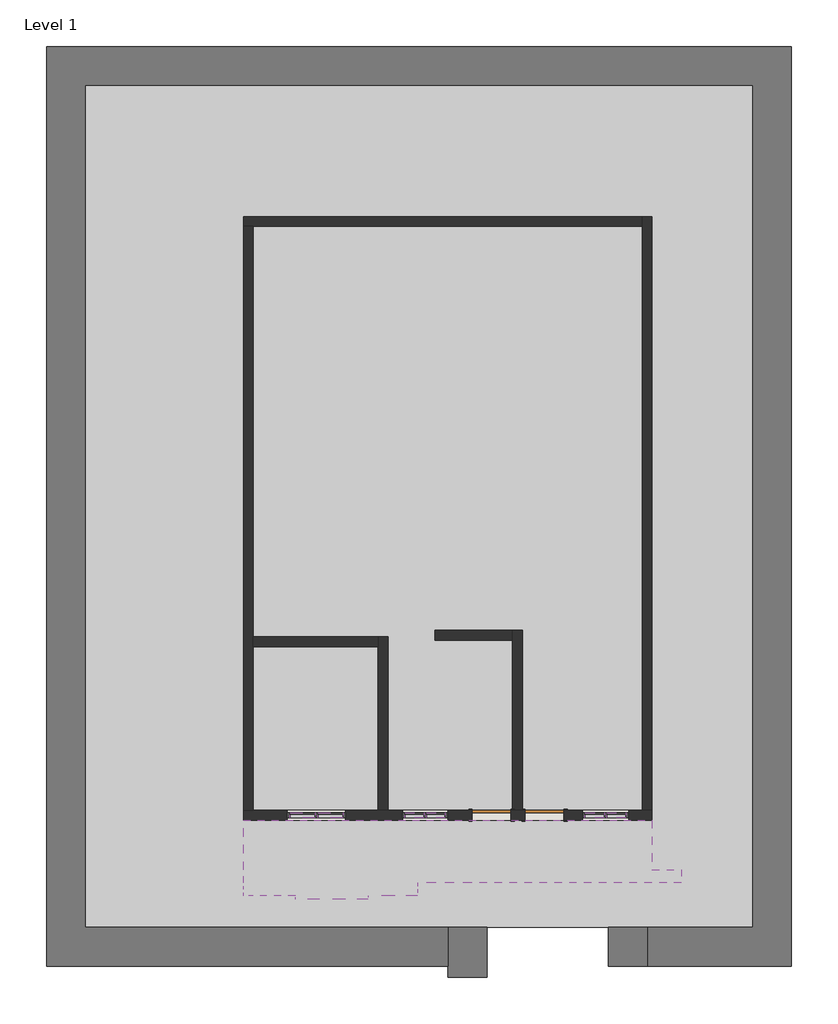
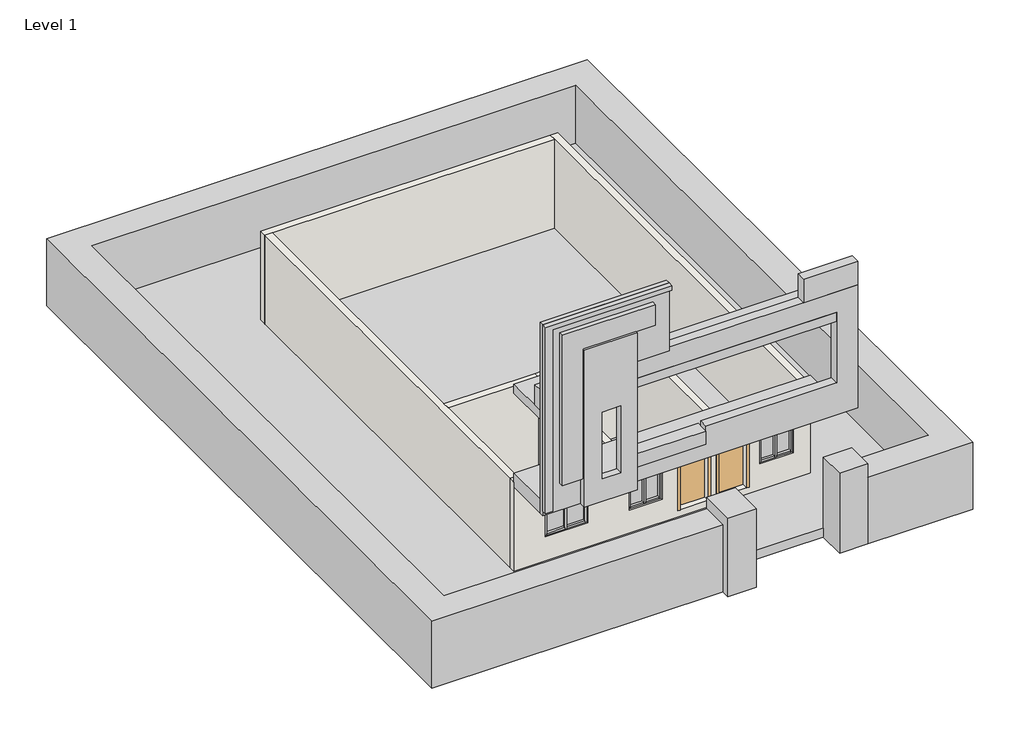
# One storey: 21 members, 8 walls, 6 plates, 3 proxies, 2 doors.
"""IFC4 building model written with IfcOpenShell, lengths in millimetres."""

from ifc_helpers import new_model, si_unit, origin, origin_with_axes, place, context, project, spatial, polyline, outline, extrude, faceted_brep, transform, mapped, element, save
from components import generic_models_1_generic_models_1_a3900748, generic_models_2_generic_models_2_88d393e9, generic_models_3_generic_models_3_c69b0eb2, door_a90ba1ad, door_0ca8825f, member_e5d39754, member_25a9efec, member_dca25542, member_6fb4a552, member_194281bb, member_24084ae4, member_969ca954, member_fe23b6ba, member_92f7bfeb, system_panel_glazed_4c12f6d8, system_panel_glazed_673a7a74, system_panel_glazed_2348052a

model = new_model("IFC4")

# Units and contexts
model_context = context("Model", 3, world=origin())
ifc_project = project(units=[si_unit("LENGTHUNIT", "METRE", prefix="MILLI")], contexts=[model_context])

# Site, building, storey
site = spatial("IfcSite", under=ifc_project)
building = spatial("IfcBuilding", under=site)
storey = spatial("IfcBuildingStorey", under=building, Name="Level 1", Elevation=0.0)

# Proxies
placement = place(None, origin())
generic_models_1_generic_models_1_shape = generic_models_1_generic_models_1_a3900748(model_context)
element("IfcBuildingElementProxy", 1, Name="Generic Models 1 : Generic Models 1", ObjectType="Generic Models 1 : Generic Models 1", at=placement, inside=storey, context=model_context, shape_type="MappedRepresentation", body=[
    mapped(generic_models_1_generic_models_1_shape, transform((0.0, 0.0, 0.0), x_axis=(1.0, 0.0, 0.0), y_axis=(0.0, 1.0, 0.0), z_axis=(0.0, 0.0, 1.0))),
])
generic_models_2_generic_models_2_shape = generic_models_2_generic_models_2_88d393e9(model_context)
element("IfcBuildingElementProxy", 2, Name="Generic Models 2 : Generic Models 2", ObjectType="Generic Models 2 : Generic Models 2", at=placement, inside=storey, context=model_context, shape_type="MappedRepresentation", body=[
    mapped(generic_models_2_generic_models_2_shape, transform((0.0, 0.0, 0.0), x_axis=(1.0, 0.0, 0.0), y_axis=(0.0, 1.0, 0.0), z_axis=(0.0, 0.0, 1.0))),
])
generic_models_3_generic_models_3_shape = generic_models_3_generic_models_3_c69b0eb2(model_context)
element("IfcBuildingElementProxy", 3, Name="Generic Models 3 : Generic Models 3", ObjectType="Generic Models 3 : Generic Models 3", at=placement, inside=storey, context=model_context, shape_type="MappedRepresentation", body=[
    mapped(generic_models_3_generic_models_3_shape, transform((0.0, 0.0, 0.0), x_axis=(1.0, 0.0, 0.0), y_axis=(0.0, 1.0, 0.0), z_axis=(0.0, 0.0, 1.0))),
])

# Doors
door_shape = door_a90ba1ad(model_context)
element("IfcDoor", 4, ObjectType="Single-Flush : 36\" x 84\"", at=placement, inside=storey, context=model_context, shape_type="MappedRepresentation", body=[
    mapped(door_shape, transform((-11559.1094994, -14629.3805842, 228.6), x_axis=(-1.0, 0.0, 0.0), y_axis=(0.0, -1.0, 0.0), z_axis=(0.0, 0.0, 1.0))),
])
door_2_shape = door_0ca8825f(model_context)
element("IfcDoor", 5, ObjectType="Single-Flush : 36\" x 84\"", at=placement, inside=storey, context=model_context, shape_type="MappedRepresentation", body=[
    mapped(door_2_shape, transform((-12803.7094994, -14629.3805842, 228.6), x_axis=(1.0, 0.0, 0.0), y_axis=(0.0, 1.0, 0.0), z_axis=(0.0, 0.0, 1.0))),
])

# Members
member_shape = member_e5d39754(model_context)
element("IfcMember", 6, ObjectType="Rectangular Mullion : 2.5\" x 5\" rectangular", at=placement, inside=storey, context=model_context, shape_type="MappedRepresentation", body=[
    mapped(member_shape, transform((-16950.2594994, -14629.3805842, 2460.3329458), x_axis=(0.0, 0.0, 1.0), y_axis=(0.0, -1.0, 0.0), z_axis=(1.0, 0.0, 0.0))),
])
element("IfcMember", 7, ObjectType="Rectangular Mullion : 2.5\" x 5\" rectangular", at=placement, inside=storey, context=model_context, shape_type="MappedRepresentation", body=[
    mapped(member_shape, transform((-16296.2094994, -14629.3805842, 2460.3329458), x_axis=(0.0, 0.0, 1.0), y_axis=(0.0, -1.0, 0.0), z_axis=(1.0, 0.0, 0.0))),
])
member_2_shape = member_25a9efec(model_context)
element("IfcMember", 8, ObjectType="Rectangular Mullion : 2.5\" x 5\" rectangular", at=placement, inside=storey, context=model_context, shape_type="MappedRepresentation", body=[
    mapped(member_2_shape, transform((-16918.5094994, -14629.3805842, 816.0272948), x_axis=(1.0, 0.0, 0.0), y_axis=(0.0, -1.0, 0.0), z_axis=(0.0, 0.0, -1.0))),
])
element("IfcMember", 9, ObjectType="Rectangular Mullion : 2.5\" x 5\" rectangular", at=placement, inside=storey, context=model_context, shape_type="MappedRepresentation", body=[
    mapped(member_shape, transform((-16886.7594994, -14629.3805842, 816.0272948), x_axis=(0.0, 0.0, -1.0), y_axis=(0.0, -1.0, 0.0), z_axis=(-1.0, 0.0, 0.0))),
])
element("IfcMember", 10, ObjectType="Rectangular Mullion : 2.5\" x 5\" rectangular", at=placement, inside=storey, context=model_context, shape_type="MappedRepresentation", body=[
    mapped(member_shape, transform((-17540.8094994, -14629.3805842, 816.0272948), x_axis=(0.0, 0.0, -1.0), y_axis=(0.0, -1.0, 0.0), z_axis=(-1.0, 0.0, 0.0))),
])
member_3_shape = member_dca25542(model_context)
element("IfcMember", 11, ObjectType="Rectangular Mullion : 2.5\" x 5\" rectangular", at=placement, inside=storey, context=model_context, shape_type="MappedRepresentation", body=[
    mapped(member_3_shape, transform((-17604.3094994, -14629.3805842, 2460.3329458), x_axis=(-1.0, 0.0, 0.0), y_axis=(0.0, -1.0, 0.0), z_axis=(0.0, 0.0, 1.0))),
])
element("IfcMember", 12, ObjectType="Rectangular Mullion : 2.5\" x 5\" rectangular", at=placement, inside=storey, context=model_context, shape_type="MappedRepresentation", body=[
    mapped(member_3_shape, transform((-16232.7094994, -14629.3805842, 816.0272948), x_axis=(1.0, 0.0, 0.0), y_axis=(0.0, -1.0, 0.0), z_axis=(0.0, 0.0, -1.0))),
])
member_4_shape = member_6fb4a552(model_context)
element("IfcMember", 13, ObjectType="Rectangular Mullion : 2.5\" x 5\" rectangular", at=placement, inside=storey, context=model_context, shape_type="MappedRepresentation", body=[
    mapped(member_4_shape, transform((-14397.5594994, -14629.3805842, 2430.1873422), x_axis=(0.0, 0.0, 1.0), y_axis=(0.0, -1.0, 0.0), z_axis=(1.0, 0.0, 0.0))),
])
element("IfcMember", 14, ObjectType="Rectangular Mullion : 2.5\" x 5\" rectangular", at=placement, inside=storey, context=model_context, shape_type="MappedRepresentation", body=[
    mapped(member_4_shape, transform((-13895.9094994, -14629.3805842, 2430.1873422), x_axis=(0.0, 0.0, 1.0), y_axis=(0.0, -1.0, 0.0), z_axis=(1.0, 0.0, 0.0))),
])
member_5_shape = member_194281bb(model_context)
element("IfcMember", 15, ObjectType="Rectangular Mullion : 2.5\" x 5\" rectangular", at=placement, inside=storey, context=model_context, shape_type="MappedRepresentation", body=[
    mapped(member_5_shape, transform((-14365.8094994, -14629.3805842, 785.4534866), x_axis=(1.0, 0.0, 0.0), y_axis=(0.0, -1.0, 0.0), z_axis=(0.0, 0.0, -1.0))),
])
element("IfcMember", 16, ObjectType="Rectangular Mullion : 2.5\" x 5\" rectangular", at=placement, inside=storey, context=model_context, shape_type="MappedRepresentation", body=[
    mapped(member_4_shape, transform((-14334.0594994, -14629.3805842, 785.4534866), x_axis=(0.0, 0.0, -1.0), y_axis=(0.0, -1.0, 0.0), z_axis=(-1.0, 0.0, 0.0))),
])
element("IfcMember", 17, ObjectType="Rectangular Mullion : 2.5\" x 5\" rectangular", at=placement, inside=storey, context=model_context, shape_type="MappedRepresentation", body=[
    mapped(member_4_shape, transform((-14835.7094994, -14629.3805842, 785.4534866), x_axis=(0.0, 0.0, -1.0), y_axis=(0.0, -1.0, 0.0), z_axis=(-1.0, 0.0, 0.0))),
])
member_6_shape = member_24084ae4(model_context)
element("IfcMember", 18, ObjectType="Rectangular Mullion : 2.5\" x 5\" rectangular", at=placement, inside=storey, context=model_context, shape_type="MappedRepresentation", body=[
    mapped(member_6_shape, transform((-14899.2094994, -14629.3805842, 2430.1873422), x_axis=(-1.0, 0.0, 0.0), y_axis=(0.0, -1.0, 0.0), z_axis=(0.0, 0.0, 1.0))),
])
element("IfcMember", 19, ObjectType="Rectangular Mullion : 2.5\" x 5\" rectangular", at=placement, inside=storey, context=model_context, shape_type="MappedRepresentation", body=[
    mapped(member_6_shape, transform((-13832.4094994, -14629.3805842, 785.4534866), x_axis=(1.0, 0.0, 0.0), y_axis=(0.0, -1.0, 0.0), z_axis=(0.0, 0.0, -1.0))),
])
member_7_shape = member_969ca954(model_context)
element("IfcMember", 20, ObjectType="Rectangular Mullion : 2.5\" x 5\" rectangular", at=placement, inside=storey, context=model_context, shape_type="MappedRepresentation", body=[
    mapped(member_7_shape, transform((-10155.7594994, -14629.3805842, 2382.0013914), x_axis=(0.0, 0.0, 1.0), y_axis=(0.0, -1.0, 0.0), z_axis=(1.0, 0.0, 0.0))),
])
element("IfcMember", 21, ObjectType="Rectangular Mullion : 2.5\" x 5\" rectangular", at=placement, inside=storey, context=model_context, shape_type="MappedRepresentation", body=[
    mapped(member_7_shape, transform((-9641.4094994, -14629.3805842, 2382.0013914), x_axis=(0.0, 0.0, 1.0), y_axis=(0.0, -1.0, 0.0), z_axis=(1.0, 0.0, 0.0))),
])
member_8_shape = member_fe23b6ba(model_context)
element("IfcMember", 22, ObjectType="Rectangular Mullion : 2.5\" x 5\" rectangular", at=placement, inside=storey, context=model_context, shape_type="MappedRepresentation", body=[
    mapped(member_8_shape, transform((-10124.0094994, -14629.3805842, 889.778584), x_axis=(1.0, 0.0, 0.0), y_axis=(0.0, -1.0, 0.0), z_axis=(0.0, 0.0, -1.0))),
])
element("IfcMember", 23, ObjectType="Rectangular Mullion : 2.5\" x 5\" rectangular", at=placement, inside=storey, context=model_context, shape_type="MappedRepresentation", body=[
    mapped(member_7_shape, transform((-10092.2594994, -14629.3805842, 889.778584), x_axis=(0.0, 0.0, -1.0), y_axis=(0.0, -1.0, 0.0), z_axis=(-1.0, 0.0, 0.0))),
])
element("IfcMember", 24, ObjectType="Rectangular Mullion : 2.5\" x 5\" rectangular", at=placement, inside=storey, context=model_context, shape_type="MappedRepresentation", body=[
    mapped(member_7_shape, transform((-10606.6094994, -14629.3805842, 889.778584), x_axis=(0.0, 0.0, -1.0), y_axis=(0.0, -1.0, 0.0), z_axis=(-1.0, 0.0, 0.0))),
])
member_9_shape = member_92f7bfeb(model_context)
element("IfcMember", 25, ObjectType="Rectangular Mullion : 2.5\" x 5\" rectangular", at=placement, inside=storey, context=model_context, shape_type="MappedRepresentation", body=[
    mapped(member_9_shape, transform((-10670.1094994, -14629.3805842, 2382.0013914), x_axis=(-1.0, 0.0, 0.0), y_axis=(0.0, -1.0, 0.0), z_axis=(0.0, 0.0, 1.0))),
])
element("IfcMember", 26, ObjectType="Rectangular Mullion : 2.5\" x 5\" rectangular", at=placement, inside=storey, context=model_context, shape_type="MappedRepresentation", body=[
    mapped(member_9_shape, transform((-9577.9094994, -14629.3805842, 889.778584), x_axis=(1.0, 0.0, 0.0), y_axis=(0.0, -1.0, 0.0), z_axis=(0.0, 0.0, -1.0))),
])

# Plates
system_panel_glazed_shape = system_panel_glazed_4c12f6d8(model_context)
element("IfcPlate", 27, ObjectType="System Panel : Glazed", at=placement, inside=storey, context=model_context, shape_type="MappedRepresentation", body=[
    mapped(system_panel_glazed_shape, transform((-17245.5344994, -14629.3805842, 879.5272948), x_axis=(1.0, 0.0, 0.0), y_axis=(0.0, 1.0, 0.0), z_axis=(0.0, 0.0, 1.0))),
])
element("IfcPlate", 28, ObjectType="System Panel : Glazed", at=placement, inside=storey, context=model_context, shape_type="MappedRepresentation", body=[
    mapped(system_panel_glazed_shape, transform((-16591.4844994, -14629.3805842, 879.5272948), x_axis=(1.0, 0.0, 0.0), y_axis=(0.0, 1.0, 0.0), z_axis=(0.0, 0.0, 1.0))),
])
system_panel_glazed_2_shape = system_panel_glazed_673a7a74(model_context)
element("IfcPlate", 29, ObjectType="System Panel : Glazed", at=placement, inside=storey, context=model_context, shape_type="MappedRepresentation", body=[
    mapped(system_panel_glazed_2_shape, transform((-14616.6344994, -14629.3805842, 848.9534866), x_axis=(1.0, 0.0, 0.0), y_axis=(0.0, 1.0, 0.0), z_axis=(0.0, 0.0, 1.0))),
])
element("IfcPlate", 30, ObjectType="System Panel : Glazed", at=placement, inside=storey, context=model_context, shape_type="MappedRepresentation", body=[
    mapped(system_panel_glazed_2_shape, transform((-14114.9844994, -14629.3805842, 848.9534866), x_axis=(1.0, 0.0, 0.0), y_axis=(0.0, 1.0, 0.0), z_axis=(0.0, 0.0, 1.0))),
])
system_panel_glazed_3_shape = system_panel_glazed_2348052a(model_context)
element("IfcPlate", 31, ObjectType="System Panel : Glazed", at=placement, inside=storey, context=model_context, shape_type="MappedRepresentation", body=[
    mapped(system_panel_glazed_3_shape, transform((-10381.1844994, -14629.3805842, 953.278584), x_axis=(1.0, 0.0, 0.0), y_axis=(0.0, 1.0, 0.0), z_axis=(0.0, 0.0, 1.0))),
])
element("IfcPlate", 32, ObjectType="System Panel : Glazed", at=placement, inside=storey, context=model_context, shape_type="MappedRepresentation", body=[
    mapped(system_panel_glazed_3_shape, transform((-9866.8344994, -14629.3805842, 953.278584), x_axis=(1.0, 0.0, 0.0), y_axis=(0.0, 1.0, 0.0), z_axis=(0.0, 0.0, 1.0))),
])

# Walls
element("IfcWall", 33, ObjectType="9\"", at=placement, inside=storey, context=model_context, shape_type="Brep", body=[
    faceted_brep([(-18633.0094994, -14743.6805842, 0.0), (-9031.8094994, -14743.6805842, 0.0), (-9031.8094994, -14743.6805842, 3048.0), (-18633.0094994, -14743.6805842, 3048.0), (-11101.9094994, -14743.6805842, 228.6), (-12016.3094994, -14743.6805842, 228.6), (-12016.3094994, -14743.6805842, 2362.2), (-11101.9094994, -14743.6805842, 2362.2), (-13260.9094994, -14743.6805842, 228.6), (-13260.9094994, -14743.6805842, 2362.2), (-12346.5094994, -14743.6805842, 2362.2), (-12346.5094994, -14743.6805842, 228.6), (-10670.1094994, -14743.6805842, 889.778584), (-10670.1094994, -14743.6805842, 2382.0013914), (-9577.9094994, -14743.6805842, 2382.0013914), (-9577.9094994, -14743.6805842, 889.778584), (-14899.2094994, -14743.6805842, 785.4534866), (-14899.2094994, -14743.6805842, 2430.1873422), (-13832.4094994, -14743.6805842, 2430.1873422), (-13832.4094994, -14743.6805842, 785.4534866), (-17604.3094994, -14743.6805842, 816.0272948), (-17604.3094994, -14743.6805842, 2460.3329458), (-16232.7094994, -14743.6805842, 2460.3329458), (-16232.7094994, -14743.6805842, 816.0272948), (-9031.8094994, -14515.0805842, 0.0), (-9260.4094994, -14515.0805842, 0.0), (-12079.8094994, -14515.0805842, 0.0), (-12308.4094994, -14515.0805842, 0.0), (-15242.1094994, -14515.0805842, 0.0), (-15470.7094994, -14515.0805842, 0.0), (-18404.4094994, -14515.0805842, 0.0), (-18633.0094994, -14515.0805842, 0.0), (-18633.0094994, -14515.0805842, 3048.0), (-18404.4094994, -14515.0805842, 3048.0), (-15470.7094994, -14515.0805842, 3048.0), (-15242.1094994, -14515.0805842, 3048.0), (-12308.4094994, -14515.0805842, 3048.0), (-12079.8094994, -14515.0805842, 3048.0), (-9260.4094994, -14515.0805842, 3048.0), (-9031.8094994, -14515.0805842, 3048.0), (-11101.9094994, -14515.0805842, 228.6), (-11101.9094994, -14515.0805842, 2362.2), (-12016.3094994, -14515.0805842, 2362.2), (-12016.3094994, -14515.0805842, 228.6), (-13260.9094994, -14515.0805842, 228.6), (-12346.5094994, -14515.0805842, 228.6), (-12346.5094994, -14515.0805842, 2362.2), (-13260.9094994, -14515.0805842, 2362.2), (-10670.1094994, -14515.0805842, 2382.0013914), (-10670.1094994, -14515.0805842, 889.778584), (-9577.9094994, -14515.0805842, 889.778584), (-9577.9094994, -14515.0805842, 2382.0013914), (-14899.2094994, -14515.0805842, 2430.1873422), (-14899.2094994, -14515.0805842, 785.4534866), (-13832.4094994, -14515.0805842, 785.4534866), (-13832.4094994, -14515.0805842, 2430.1873422), (-17604.3094994, -14515.0805842, 2460.3329458), (-17604.3094994, -14515.0805842, 816.0272948), (-16232.7094994, -14515.0805842, 816.0272948), (-16232.7094994, -14515.0805842, 2460.3329458)], [[[0, 1, 2, 3], [4, 5, 6, 7], [8, 9, 10, 11], [12, 13, 14, 15], [16, 17, 18, 19], [20, 21, 22, 23]], [[24, 25, 26, 27, 28, 29, 30, 31, 32, 33, 34, 35, 36, 37, 38, 39], [40, 41, 42, 43], [44, 45, 46, 47], [48, 49, 50, 51], [52, 53, 54, 55], [56, 57, 58, 59]], [[1, 0, 31, 30, 29, 28, 27, 26, 25, 24]], [[3, 2, 39, 38, 37, 36, 35, 34, 33, 32]], [[2, 1, 24, 39]], [[0, 3, 32, 31]], [[5, 4, 40, 43]], [[6, 5, 43, 42]], [[7, 6, 42, 41]], [[4, 7, 41, 40]], [[45, 44, 8, 11]], [[46, 45, 11, 10]], [[47, 46, 10, 9]], [[44, 47, 9, 8]], [[12, 49, 48, 13]], [[13, 48, 51, 14]], [[14, 51, 50, 15]], [[49, 12, 15, 50]], [[52, 17, 16, 53]], [[17, 52, 55, 18]], [[18, 55, 54, 19]], [[53, 16, 19, 54]], [[56, 21, 20, 57]], [[21, 56, 59, 22]], [[22, 59, 58, 23]], [[57, 20, 23, 58]]]),
])
element("IfcWall", 34, ObjectType="9\"", at=placement, inside=storey, context=model_context, shape_type="Brep", body=[
    faceted_brep([(-9031.8094994, -14515.0805842, 0.0), (-9031.8094994, -570.4805842, 0.0), (-9031.8094994, -570.4805842, 3048.0), (-9031.8094994, -14515.0805842, 3048.0), (-9260.4094994, -14515.0805842, 0.0), (-9260.4094994, -14515.0805842, 3048.0), (-9260.4094994, -799.0805842, 3048.0), (-9260.4094994, -570.4805842, 3048.0), (-9260.4094994, -570.4805842, 0.0), (-9260.4094994, -799.0805842, 0.0)], [[[0, 1, 2, 3]], [[4, 5, 6, 7, 8, 9]], [[1, 0, 4, 9, 8]], [[3, 2, 7, 6, 5]], [[0, 3, 5, 4]], [[2, 1, 8, 7]]]),
])
element("IfcWall", 35, ObjectType="9\"", at=placement, inside=storey, context=model_context, shape_type="Brep", body=[
    faceted_brep([(-9260.4094994, -570.4805842, 0.0), (-18633.0094994, -570.4805842, 0.0), (-18633.0094994, -570.4805842, 3048.0), (-9260.4094994, -570.4805842, 3048.0), (-9260.4094994, -799.0805842, 0.0), (-9260.4094994, -799.0805842, 3048.0), (-18404.4094994, -799.0805842, 3048.0), (-18633.0094994, -799.0805842, 3048.0), (-18633.0094994, -799.0805842, 0.0), (-18404.4094994, -799.0805842, 0.0)], [[[0, 1, 2, 3]], [[4, 5, 6, 7, 8, 9]], [[1, 0, 4, 9, 8]], [[3, 2, 7, 6, 5]], [[0, 3, 5, 4]], [[2, 1, 8, 7]]]),
])
element("IfcWall", 36, ObjectType="9\"", at=placement, inside=storey, context=model_context, shape_type="Brep", body=[
    faceted_brep([(-18633.0094994, -799.0805842, 0.0), (-18633.0094994, -14515.0805842, 0.0), (-18633.0094994, -14515.0805842, 3048.0), (-18633.0094994, -799.0805842, 3048.0), (-18404.4094994, -799.0805842, 0.0), (-18404.4094994, -799.0805842, 3048.0), (-18404.4094994, -10438.3805842, 3048.0), (-18404.4094994, -10666.9805842, 3048.0), (-18404.4094994, -14515.0805842, 3048.0), (-18404.4094994, -14515.0805842, 0.0), (-18404.4094994, -10666.9805842, 0.0), (-18404.4094994, -10438.3805842, 0.0)], [[[0, 1, 2, 3]], [[4, 5, 6, 7, 8, 9, 10, 11]], [[1, 0, 4, 11, 10, 9]], [[3, 2, 8, 7, 6, 5]], [[0, 3, 5, 4]], [[2, 1, 9, 8]]]),
])
element("IfcWall", 37, ObjectType="9\"", at=placement, inside=storey, context=model_context, shape_type="Brep", body=[
    faceted_brep([(-15242.1094994, -14515.0805842, 0.0), (-15242.1094994, -10438.3805842, 0.0), (-15242.1094994, -10438.3805842, 3048.0), (-15242.1094994, -14515.0805842, 3048.0), (-15470.7094994, -14515.0805842, 0.0), (-15470.7094994, -14515.0805842, 3048.0), (-15470.7094994, -10666.9805842, 3048.0), (-15470.7094994, -10438.3805842, 3048.0), (-15470.7094994, -10438.3805842, 0.0), (-15470.7094994, -10666.9805842, 0.0)], [[[0, 1, 2, 3]], [[4, 5, 6, 7, 8, 9]], [[1, 0, 4, 9, 8]], [[3, 2, 7, 6, 5]], [[0, 3, 5, 4]], [[2, 1, 8, 7]]]),
])
element("IfcWall", 38, ObjectType="9\"", at=placement, inside=storey, context=model_context, shape_type="SweptSolid", body=[
    extrude(outline(polyline([(-18404.4094994, -10438.3805842), (-15470.7094994, -10438.3805842), (-15470.7094994, -10666.9805842), (-18404.4094994, -10666.9805842), (-18404.4094994, -10438.3805842)])), origin_with_axes(), (0.0, 0.0, 1.0), 3048.0),
])
element("IfcWall", 39, ObjectType="9\"", at=placement, inside=storey, context=model_context, shape_type="Brep", body=[
    faceted_brep([(-12079.8094994, -14515.0805842, 0.0), (-12079.8094994, -10285.9805842, 0.0), (-12079.8094994, -10285.9805842, 3048.0), (-12079.8094994, -14515.0805842, 3048.0), (-12308.4094994, -14515.0805842, 0.0), (-12308.4094994, -14515.0805842, 3048.0), (-12308.4094994, -10514.5805842, 3048.0), (-12308.4094994, -10285.9805842, 3048.0), (-12308.4094994, -10285.9805842, 0.0), (-12308.4094994, -10514.5805842, 0.0)], [[[0, 1, 2, 3]], [[4, 5, 6, 7, 8, 9]], [[1, 0, 4, 9, 8]], [[3, 2, 7, 6, 5]], [[0, 3, 5, 4]], [[2, 1, 8, 7]]]),
])
element("IfcWall", 40, ObjectType="9\"", at=placement, inside=storey, context=model_context, shape_type="SweptSolid", body=[
    extrude(outline(polyline([(-14137.2094994, -10285.9805842), (-12308.4094994, -10285.9805842), (-12308.4094994, -10514.5805842), (-14137.2094994, -10514.5805842), (-14137.2094994, -10285.9805842)])), origin_with_axes(), (0.0, 0.0, 1.0), 3048.0),
])

save(model, "model.ifc")

# Revit data of these elements
# Type "Single-Flush : 36\" x 84\""
#   Type Mark = "1"
#   Construction Type Id = "MDOOR"
#   Assembly Code = "C1020"
#   Analytic Construction = "Metal"
#   Thickness = 0' - 2"
#   Heat Transfer Coefficient (U) = 0.651978 BTU/(h·ft²·°F)
#   Height = 7' - 0"
#   Trim Projection Ext = 0' - 1"
#   Trim Projection Int = 0' - 1"
#   Trim Width = 0' - 3"
#   Width = 3' - 0"
#   Define Thermal Properties by = 1
#   Define Thermal Properties by = 1
#   Door Material = Door - Panel
#   Frame Material = Door - Frame
#   Visual Light Transmittance = 0
#   Solar Heat Gain Coefficient = 0
#   Function = (empty or 0)
#   Wall Closure = (empty or 0)
# Type "Rectangular Mullion : 2.5\" x 5\" rectangular"
#   built-in parameter 1007304 = 0.416667 (stored number, unit not read)
#   built-in parameter 1007301 = 0.104167 (stored number, unit not read)
#   built-in parameter 1007300 = 0.104167 (stored number, unit not read)
# Type "System Panel : Glazed"
#   Construction Type Id = "GSP4R"
#   Analytic Construction = "1/8 in Pilkington single glazing"
#   Visual Light Transmittance = 0.9
#   Solar Heat Gain Coefficient = 0.86
#   Heat Transfer Coefficient (U) = 1.18115 BTU/(h·ft²·°F)
#   Define Thermal Properties by = 1
# Type "9\""
#   Assembly Code = "B2010"
#   Layers, outside or top first: 0' - 9" no material (function 1)
# Element 1 (IfcBuildingElementProxy, "Generic Models 1 : Generic Models 1")
#   Phase Created = New Construction
# Element 2 (IfcBuildingElementProxy, "Generic Models 2 : Generic Models 2")
#   Phase Created = New Construction
# Element 3 (IfcBuildingElementProxy, "Generic Models 3 : Generic Models 3")
#   Phase Created = New Construction
# Elements 4, 5 (IfcDoor, "Single-Flush : 36\" x 84\"")
#   Phase Created = New Construction
#   Materials on its faces: "Door - Frame", "Door - Panel"
# Elements 6, 7, 8, 9, 10, 11, 12, 13, 14, 15, 16, 17, 18, 19, 20, 21, 22, 23, 24, 25, 26 (IfcMember, "Rectangular Mullion : 2.5\" x 5\" rectangular")
#   Phase Created = New Construction
#   Materials on its faces: "Aluminum"
# Elements 27, 28, 29, 30, 31, 32 (IfcPlate, "System Panel : Glazed")
#   Phase Created = New Construction
#   Materials on its faces: "Glass"
# Elements 33, 34, 35, 36, 37, 38, 39, 40 (IfcWall, "9\"")
#   Top Offset = 0' - 0"
#   Base Offset = 0' - 0"
#   Unconnected Height = 10' - 0"
#   wall height = 10' - 0"
#   Phase Created = New Construction
#   Base Constraint = Level 1
#   Materials on its faces: "Default Wall"
# Materials
#   "Door - Panel": class "Wood", colour RGB 210 159 95, transparency 0, Cost = 0
#   "Door - Frame": colour RGB 118 70 51, transparency 0, Cost = 0
#   "Aluminum": class "Metal", colour RGB 247 247 247, transparency 0, Description = "Aluminum 6061", Cost = 0
#   "Glass": class "Glass", colour RGB 0 128 192, transparency 0.75, Description = "Soda Lime Glass", Cost = 0
#   "Default Wall": colour RGB 128 128 128, transparency 0, Cost = 0
